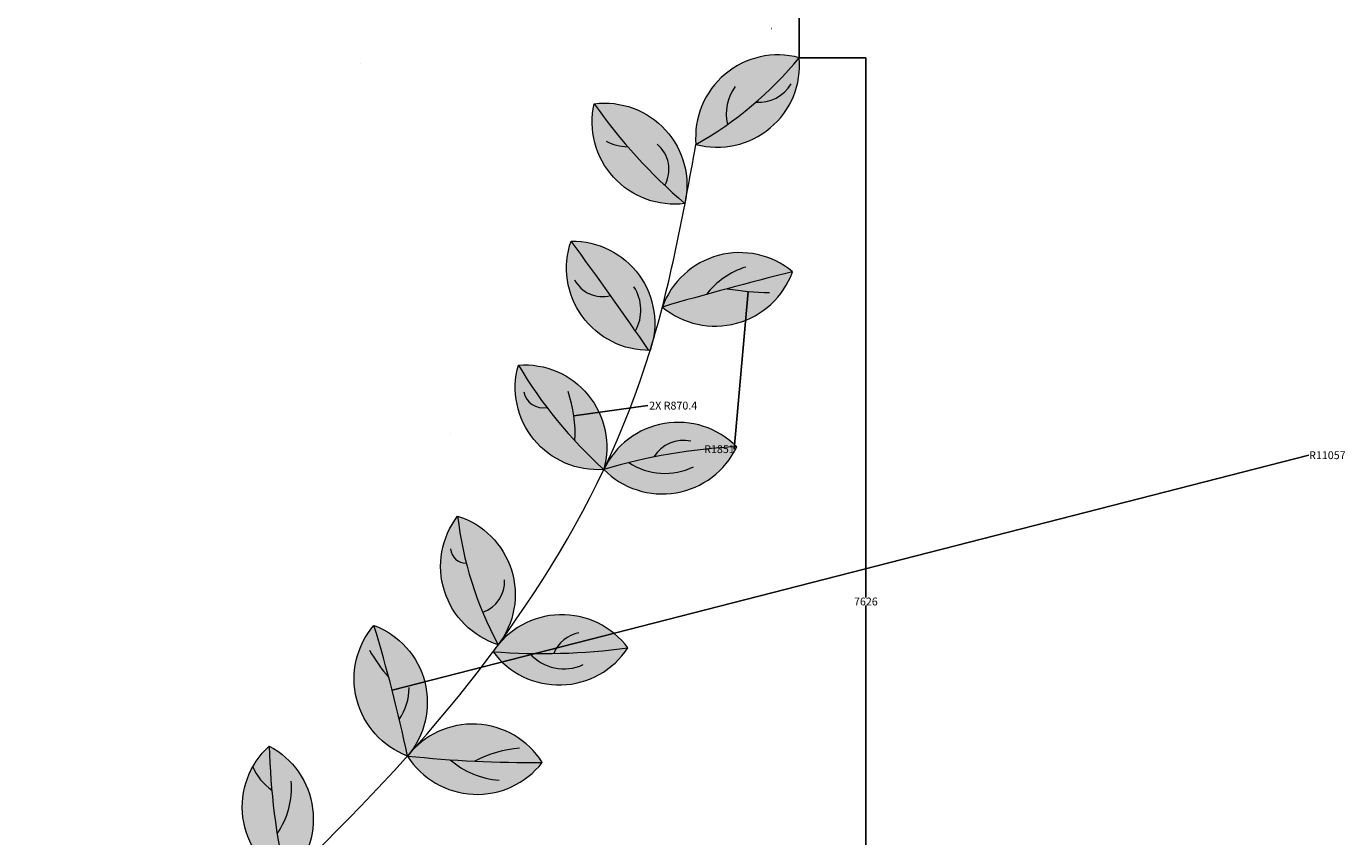
# Model space of a CAD drawing. Units: millimetres. Extents: x 8570 to 49085, y 3782 to 24863.
# Tile 14 of 15: x 39837 to 49085, y 9648 to 15329. Entities that reach past the tile are written whole.
import ezdxf

# ---------------------------------------------------------------- set-up
doc = ezdxf.new("R2010")
doc.units = ezdxf.units.MM
doc.header["$MEASUREMENT"] = 0
doc.header["$PDMODE"] = 3
for name, color, linetype, lineweight in [('A-ANNO-DIMS', 2, 'Continuous', 18), ('A-DETL-FOLI', 7, 'Continuous', 13), ('A-DETL-PATT', 3, 'Continuous', 13), ('A-DETL-STEM', 28, 'Continuous', 18)]:
    doc.layers.add(name, color=color, linetype=linetype, lineweight=lineweight)
doc.styles.get("Standard").update_dxf_attribs({"font": 'arial.ttf'})
doc.dimstyles.get("Standard").update_dxf_attribs({"dimtxt": 55, "dimasz": 0.18, "dimexe": 0.18, "dimexo": 0.0625, "dimgap": 0.09, "dimtad": 0, "dimtih": 1, "dimtoh": 1, "dimdec": 0, "dimzin": 0, "dimdsep": 46, "dimtxsty": 'Standard', "dimcen": 0.09, "dimadec": 0, "dimazin": 0, "dimtfac": 1, "dimtdec": 0, "dimtofl": 0, "dimtmove": 0, "dimatfit": 3, "dimfxl": 1, "dimtolj": 1, "dimtzin": 0, "dimarcsym": 0})

# ---------------------------------------------------------------- blocks, each defined once
blk = doc.blocks.new('*D72')
at = {"layer": 'A-ANNO-DIMS', "color": 0, "lineweight": -2, "transparency": 16777216}
for p, q in [((36229.4, 13941.8), (36229.4, 17114.8)), ((36229.6, 17114.6), (40660.1, 17114.6)), ((45255, 17114.6), (40824.5, 17114.6)), ((45255.2, 15109.6), (45255.2, 17114.8))]:
    blk.add_line(p, q, dxfattribs=at)
at = {"layer": 'A-ANNO-DIMS', "color": 0, "transparency": 16777216}
for points in [[(36229.6, 17114.7), (36229.6, 17114.6), (36229.4, 17114.6)], [(45255, 17114.7), (45255, 17114.6), (45255.2, 17114.6)]]:
    blk.add_solid(points, dxfattribs=at)
at = {"layer": 'Defpoints', "color": 0, "transparency": 16777216}
for p in [(45255.2, 17114.6), (45255.2, 15109.5), (36229.4, 13941.8)]:
    blk.add_point(p, dxfattribs=at)
at = {"layer": 'A-ANNO-DIMS', "color": 0, "transparency": 16777216, "insert": (40742.3, 17114.6), "char_height": 55, "attachment_point": 5}
blk.add_mtext('\\A1;9026', dxfattribs=at)
blk = doc.blocks.new('*D76')
at = {"layer": 'A-ANNO-DIMS', "color": 0, "lineweight": -2, "transparency": 16777216}
for p, q in [((45255.3, 15109.5), (45721.9, 15109.5)), ((45721.7, 15109.3), (45721.7, 11324.7)), ((45721.7, 7483.7), (45721.7, 11268.3)), ((39491.1, 7483.5), (45721.9, 7483.5))]:
    blk.add_line(p, q, dxfattribs=at)
at = {"layer": 'A-ANNO-DIMS', "color": 0, "transparency": 16777216}
for points in [[(45721.6, 15109.3), (45721.7, 15109.3), (45721.7, 15109.5)], [(45721.6, 7483.7), (45721.7, 7483.7), (45721.7, 7483.5)]]:
    blk.add_solid(points, dxfattribs=at)
at = {"layer": 'Defpoints', "color": 0, "transparency": 16777216}
for p in [(45255.2, 15109.5), (45721.7, 15109.5), (39491, 7483.5)]:
    blk.add_point(p, dxfattribs=at)
at = {"layer": 'A-ANNO-DIMS', "color": 0, "transparency": 16777216, "insert": (45721.7, 11296.5), "char_height": 55, "attachment_point": 5}
blk.add_mtext('\\A1;7626', dxfattribs=at)
blk = doc.blocks.new('*D95')
at = {"layer": 'A-ANNO-DIMS', "color": 0, "lineweight": -2, "transparency": 16777216}
for p, q in [((48826.8, 12322.2), (42401, 10673.8)), ((31690.9, 7926.2), (31691.1, 7926.2)), ((31691, 7926.2), (31691, 7926.3))]:
    blk.add_line(p, q, dxfattribs=at)
at = {"layer": 'A-ANNO-DIMS', "color": 0, "transparency": 16777216}
blk.add_solid([(42401, 10673.8), (42401, 10673.7), (42400.9, 10673.7)], dxfattribs=at)
at = {"layer": 'Defpoints', "color": 0, "transparency": 16777216}
for p in [(42400.9, 10673.7), (31691, 7926.2)]:
    blk.add_point(p, dxfattribs=at)
at = {"layer": 'A-ANNO-DIMS', "color": 0, "transparency": 16777216, "insert": (48956.7, 12322.2), "char_height": 55, "attachment_point": 5}
blk.add_mtext('\\A1;R11057', dxfattribs=at)
blk = doc.blocks.new('*D96')
at = {"layer": 'A-ANNO-DIMS', "color": 0, "lineweight": -2, "transparency": 16777216}
for p, q in [((42176.7, 15068.1), (42176.9, 15068.1)), ((42176.8, 15068), (42176.8, 15068.2)), ((40544.1, 4385.9), (41156.3, 8391.6)), ((40543.9, 4385.9), (40544.1, 4385.9))]:
    blk.add_line(p, q, dxfattribs=at)
at = {"layer": 'A-ANNO-DIMS', "color": 0, "transparency": 16777216}
blk.add_solid([(41156.3, 8391.6), (41156.3, 8391.6), (41156.3, 8391.7)], dxfattribs=at)
at = {"layer": 'Defpoints', "color": 0, "transparency": 16777216}
for p in [(42176.8, 15068.1), (41156.3, 8391.7)]:
    blk.add_point(p, dxfattribs=at)
at = {"layer": 'A-ANNO-DIMS', "color": 0, "transparency": 16777216, "insert": (40375.9, 4385.9), "char_height": 55, "attachment_point": 5}
blk.add_mtext('\\A1;2X R6754', dxfattribs=at)
blk = doc.blocks.new('*D98')
at = {"layer": 'A-ANNO-DIMS', "color": 0, "lineweight": -2, "transparency": 16777216}
for p, q in [((45061.3, 15314.3), (45061.3, 15314.5)), ((45061.3, 15314.4), (45061.4, 15314.4)), ((44798.9, 12364.6), (44897.3, 13470.6)), ((44798.7, 12364.6), (44798.9, 12364.6))]:
    blk.add_line(p, q, dxfattribs=at)
at = {"layer": 'A-ANNO-DIMS', "color": 0, "transparency": 16777216}
blk.add_solid([(44897.3, 13470.6), (44897.3, 13470.6), (44897.3, 13470.8)], dxfattribs=at)
at = {"layer": 'Defpoints', "color": 0, "transparency": 16777216}
for p in [(45061.3, 15314.4), (44897.3, 13470.8)]:
    blk.add_point(p, dxfattribs=at)
at = {"layer": 'A-ANNO-DIMS', "color": 0, "transparency": 16777216, "insert": (44695.5, 12364.6), "char_height": 55, "attachment_point": 5}
blk.add_mtext('\\A1;R1851', dxfattribs=at)
blk = doc.blocks.new('*D100')
at = {"layer": 'A-ANNO-DIMS', "color": 0, "lineweight": -2, "transparency": 16777216}
for p, q in [((44192.6, 12670.1), (43675.6, 12598)), ((42813.3, 12477.8), (42813.5, 12477.8)), ((42813.4, 12477.8), (42813.4, 12477.9))]:
    blk.add_line(p, q, dxfattribs=at)
at = {"layer": 'A-ANNO-DIMS', "color": 0, "transparency": 16777216}
blk.add_solid([(43675.6, 12598), (43675.6, 12598), (43675.4, 12598)], dxfattribs=at)
at = {"layer": 'Defpoints', "color": 0, "transparency": 16777216}
for p in [(43675.4, 12598), (42813.4, 12477.8)]:
    blk.add_point(p, dxfattribs=at)
at = {"layer": 'A-ANNO-DIMS', "color": 0, "transparency": 16777216, "insert": (44371.3, 12670.1), "char_height": 55, "attachment_point": 5}
blk.add_mtext('\\A1;2X R870.4', dxfattribs=at)

msp = doc.modelspace()

# ---------------------------------------------------------------- hatches: boundary and pattern name
at = {"layer": 'A-DETL-PATT'}
h = msp.add_hatch(color=256, dxfattribs=at)
h.dxf.hatch_style = 1
h.paths.add_polyline_path([(45255.2, 15109.49, 0.520567), (44530.5, 14502, 0.0921742)])
h = msp.add_hatch(color=256, dxfattribs=at)
h.dxf.hatch_style = 1
h.paths.add_polyline_path([(45255.2, 15109.49, -0.0921742), (44530.5, 14502, 0.5205671)])
h = msp.add_hatch(color=256, dxfattribs=at)
h.dxf.hatch_style = 1
h.paths.add_polyline_path([(43817.43, 14786.58, 0.520567), (44453.74, 14087.05, -0.0631799)])
h = msp.add_hatch(color=256, dxfattribs=at)
h.dxf.hatch_style = 1
edge = h.paths.add_edge_path()
edge.add_arc((46892.53, 16944.63), 3756.78, 215.060458, 229.520994)
edge.add_spline(control_points=[(44453.74, 14087.05), (44480.13, 14224.97), (44505.32, 14363.49), (44530.5, 14502)], knot_values=[8364.9516505, 8364.9516505, 8364.9516505, 8364.9516505, 8782.9420196, 8782.9420196, 8782.9420196, 8782.9420196], degree=3, periodic=0)
edge.add_arc((43890.68, 14214.04), 577.2, 351.357941, 457.290726)
h = msp.add_hatch(color=256, dxfattribs=at)
h.dxf.hatch_style = 1
h.paths.add_polyline_path([(43655.71, 13823.96, 0.5158234), (44200.99, 13057.47, 0.0070598)])
h = msp.add_hatch(color=256, dxfattribs=at)
h.dxf.hatch_style = 1
h.paths.add_polyline_path([(43655.71, 13823.96, -0.0070598), (44200.99, 13057.47, 0.0037395), (44209.63, 13057.54, 0.520567)])
h = msp.add_hatch(color=256, dxfattribs=at)
h.dxf.hatch_style = 1
h.paths.add_polyline_path([(45207.81, 13608.75, 0.520567), (44295.07, 13361.5, -0.0103411)])
h = msp.add_hatch(color=256, dxfattribs=at)
h.dxf.hatch_style = 1
h.paths.add_polyline_path([(45207.81, 13608.75, 0.0103411), (44295.07, 13361.5, 0.5205671)])
h = msp.add_hatch(color=256, dxfattribs=at)
h.dxf.hatch_style = 1
h.paths.add_polyline_path([(43285.74, 12954.22, 0.5205671), (43884.37, 12222.19, -0.0744626)])
h = msp.add_hatch(color=256, dxfattribs=at)
h.dxf.hatch_style = 1
h.paths.add_polyline_path([(43285.74, 12954.22, 0.0744626), (43884.37, 12222.19, 0.5205671)])
h = msp.add_hatch(color=256, dxfattribs=at)
h.dxf.hatch_style = 1
h.paths.add_polyline_path([(43884.37, 12222.19, -0.0616433), (44816.59, 12380.95, 0.5205671)])
h = msp.add_hatch(color=256, dxfattribs=at)
h.dxf.hatch_style = 1
h.paths.add_polyline_path([(43884.37, 12222.19, 0.520567), (44816.59, 12380.95, 0.0616433)])
h = msp.add_hatch(color=256, dxfattribs=at)
h.dxf.hatch_style = 1
h.paths.add_polyline_path([(42859.98, 11895.45, 0.520567), (43144.45, 10993.62, -0.0955481)])
h = msp.add_hatch(color=256, dxfattribs=at)
h.dxf.hatch_style = 1
edge = h.paths.add_edge_path()
edge.add_spline(control_points=[(43144.45, 10993.62), (43149.8, 11000.92), (43155.14, 11008.22), (43160.46, 11015.54)], knot_values=[4911.3561457, 4911.3561457, 4911.3561457, 4911.3561457, 4938.9064516, 4938.9064516, 4938.9064516, 4938.9064516], degree=3, periodic=0)
edge.add_arc((42686.48, 11344.94), 577.2, 325.201512, 432.507225)
edge.add_arc((45340.3, 12182.06), 2496.83, 186.591356, 208.423095)
h = msp.add_hatch(color=256, dxfattribs=at)
h.dxf.hatch_style = 1
edge = h.paths.add_edge_path()
edge.add_arc((43590.08, 10626.76), 577.2, 36.607727, 140.537696)
edge.add_spline(control_points=[(43144.45, 10993.62), (43132.42, 10977.19), (43120.32, 10960.8), (43108.16, 10944.44)], knot_values=[4849.3638092, 4849.3638092, 4849.3638092, 4849.3638092, 4911.3561457, 4911.3561457, 4911.3561457, 4911.3561457], degree=3, periodic=0)
edge.add_arc((43453.14, 15505.77), 4574.36, 265.674876, 277.540577)
h = msp.add_hatch(color=256, dxfattribs=at)
h.dxf.hatch_style = 1
h.paths.add_polyline_path([(42273.58, 11129.19, 0.5205671), (42508.56, 10213.21, 0.0213914)])
h = msp.add_hatch(color=256, dxfattribs=at)
h.dxf.hatch_style = 1
h.paths.add_polyline_path([(42273.58, 11129.19, -0.0213914), (42508.56, 10213.21, -0.0124698), (42526.74, 10235.52, 0.5048203)])
h = msp.add_hatch(color=256, dxfattribs=at)
h.dxf.hatch_style = 1
h.paths.add_polyline_path([(43108.16, 10944.44, 0.520567), (44053.42, 10970.97, -0.0518202)])
h = msp.add_hatch(color=256, dxfattribs=at)
h.dxf.hatch_style = 1
h.paths.add_polyline_path([(42526.74, 10235.52, -0.0124698), (42508.56, 10213.21, 0.0289339), (43453.1, 10167.77, 0.5048203)])
h = msp.add_hatch(color=256, dxfattribs=at)
h.dxf.hatch_style = 1
h.paths.add_polyline_path([(41539.85, 10282.96, 0.0816048), (41423.54, 10136.32, 0.1348282), (41557.06, 9974.44, -0.0171383)])
h = msp.add_hatch(color=256, dxfattribs=at)
h.dxf.hatch_style = 1
h.paths.add_polyline_path([(41539.85, 10282.96, 0.0525775), (41659.15, 9344.88, -0.0152167), (41684.42, 9369.28, 0.5013788)])
h = msp.add_hatch(color=256, dxfattribs=at)
h.dxf.hatch_style = 1
h.paths.add_polyline_path([(42508.56, 10213.21, 0.520567), (43453.1, 10167.77, -0.0289339)])
h = msp.add_hatch(color=256, dxfattribs=at)
h.dxf.hatch_style = 1
h.paths.add_polyline_path([(41423.54, 10136.32, 0.4210746), (41659.15, 9344.88, -0.0354074), (41557.06, 9974.44, -0.1348282)])

# ---------------------------------------------------------------- linework, layer by layer
at = {"layer": 'A-DETL-FOLI'}
for points in [[(44530.5, 14502, 0.5205671), (45255.2, 15109.49, 0.5205671)], [(44453.74, 14087.05, -0.5205671), (43817.43, 14786.58, -0.5205671)], [(44209.63, 13057.54, -0.5205671), (43655.71, 13823.96, -0.5205671)], [(44295.07, 13361.5, 0.520567), (45207.81, 13608.75, 0.520567)], [(43884.37, 12222.19, -0.5205671), (43285.74, 12954.22, -0.5205671)], [(43884.37, 12222.19, 0.5205671), (44816.59, 12380.95, 0.5205671)], [(43144.45, 10993.62, -0.5205671), (42859.98, 11895.45, -0.5205671)], [(43108.16, 10944.44, 0.5205671), (44053.42, 10970.97, 0.5205671)], [(42508.56, 10213.21, -0.5205671), (42273.58, 11129.19, -0.5205671)], [(42508.56, 10213.21, 0.5205671), (43453.1, 10167.77, 0.5205671)], [(41659.15, 9344.88, -0.5205671), (41539.85, 10282.96, -0.5205671)]]:
    msp.add_lwpolyline(points, format="xyb", close=True, dxfattribs=at)
for centre, radius, start, end in [((43259.18, 16754.61), 2586.6, 299.439355, 320.504599), ((45061.29, 14715.4), 318.77, 143.014841, 193.372003), ((44967.71, 15064.13), 267.7, 266.177281, 329.039302), ((46892.53, 16944.63), 3756.78, 215.060458, 229.520994), ((44063.32, 14834.72), 349.86, 242.373848, 268.287524), ((44110.74, 14326.98), 230.45, 330.782563, 50.239386), ((16787.02, -5867.96), 33312.13, 34.619535, 36.23749), ((50728, -8578.48), 22863.63, 103.971549, 106.341464), ((45045.6, 13108.73), 558.08, 107.22426, 142.344654), ((43873.8, 13655.01), 219.96, 207.580175, 285.088667), ((43844.51, 13339.47), 299.94, 330.886086, 33.127881), ((45061.34, 15314.37), 1850.87, 260.320947, 269.509672), ((46029.14, 14586.9), 3192.47, 210.758257, 227.792395), ((43460.71, 12793.77), 139.85, 190.917783, 280.648361), ((42813.38, 12477.85), 870.37, 356.380694, 19.487396), ((44442.82, 12182.96), 242.64, 77.562806, 148.420752), ((44991.89, 8535.26), 3849.69, 92.609965, 106.719724), ((44312.06, 12654.63), 460, 236.673555, 296.069992), ((45340.3, 12182.06), 2496.83, 186.591356, 208.423095), ((42918.88, 11674.62), 108.88, 184.996226, 270.97743), ((42961.4, 11437.72), 228.57, 288.948724, 2.800617), ((31690.99, 7926.25), 11056.67, 11.937248, 16.839041), ((43756.08, 10840.38), 240.93, 100.974089, 157.618816), ((43130.73, 11432.05), 1007.16, 208.180992, 221.585722), ((43453.14, 15505.77), 4574.36, 265.674876, 277.540577), ((43605, 11142.55), 318.74, 221.283103, 295.080001), ((42118.78, 10695.59), 401.41, 325.85536, 359.694647), ((46047.63, 10379.64), 4508.82, 181.228633, 193.267432), ((43359.77, 9455.11), 815.46, 94.623229, 117.742552), ((43373.1, 18344.88), 8177.5, 263.931196, 270.56051), ((43194.21, 10632), 589.63, 229.003412, 265.710705), ((41785.01, 10298.45), 396.17, 204.157103, 234.872231), ((41130.3, 9990.38), 565.03, 325.354259, 4.717429)]:
    msp.add_arc(centre, radius, start, end, dxfattribs=at)
at = {"layer": 'A-DETL-STEM'}
msp.add_open_spline([(39491, 7483.5), (41497.86, 9125.36), (43912.02, 11100.44), (44441.22, 14010.96), (44530.5, 14502)], degree=3, knots=[0, 0, 0, 0, 7301.1442939, 8782.9420196, 8782.9420196, 8782.9420196, 8782.9420196], dxfattribs=at)

# ---------------------------------------------------------------- dimensions: what is measured, and where the dimension line sits
at = {"layer": 'A-ANNO-DIMS'}
dim = msp.add_linear_dim(base=(45255.2, 17114.63), p1=(36229.45, 13941.76), p2=(45255.2, 15109.49), dimstyle='Standard', override={"dimdec": 0, "dimlfac": 1, "dimrnd": 0, "dimzin": 0, "dimdsep": 46, "dimlunit": 2}, dxfattribs=at)
dim.commit()
dim.dimension.update_dxf_attribs({"geometry": '*D72', "text_midpoint": (40742.32, 17114.63)})
for center, mpoint, picture, middle in [((45061.34, 15314.37), (44897.3, 13470.78), '*D98', (44695.48, 12364.63)), ((31690.99, 7926.25), (42400.86, 10673.71), '*D95', (48826.79, 12322.19))]:
    dim = msp.add_radius_dim(center=center, mpoint=mpoint, dimstyle='Standard', override={"dimdec": 0, "dimlfac": 1, "dimrnd": 0, "dimzin": 0, "dimdsep": 46, "dimlunit": 2}, dxfattribs=at)
    dim.commit()
    dim.dimension.update_dxf_attribs({"geometry": picture, "text_midpoint": middle, "dimtype": 164})
dim = msp.add_linear_dim(base=(45721.68, 15109.49), p1=(39491, 7483.5), p2=(45255.2, 15109.49), angle=90, dimstyle='Standard', override={"dimdec": 0, "dimlfac": 1, "dimrnd": 0, "dimzin": 0, "dimdsep": 46, "dimlunit": 2}, dxfattribs=at)
dim.commit()
dim.dimension.update_dxf_attribs({"geometry": '*D76', "text_midpoint": (45721.68, 11296.49)})
for center, mpoint, override, picture, middle in [((42176.8, 15068.1), (41156.34, 8391.74), {"dimdec": 0, "dimlfac": 1, "dimrnd": 0, "dimzin": 0, "dimdsep": 46, "dimlunit": 2}, '*D96', (40375.91, 4385.92)), ((42813.38, 12477.85), (43675.42, 12597.99), {"dimdec": 1, "dimlfac": 1, "dimrnd": 0, "dimzin": 0, "dimdsep": 46, "dimlunit": 2}, '*D100', (44192.64, 12670.07))]:
    dim = msp.add_radius_dim(center=center, mpoint=mpoint, text='2X <>', dimstyle='Standard', override=override, dxfattribs=at)
    dim.commit()
    dim.dimension.update_dxf_attribs({"geometry": picture, "text_midpoint": middle, "dimtype": 164})

doc.saveas('drawing.dxf')
